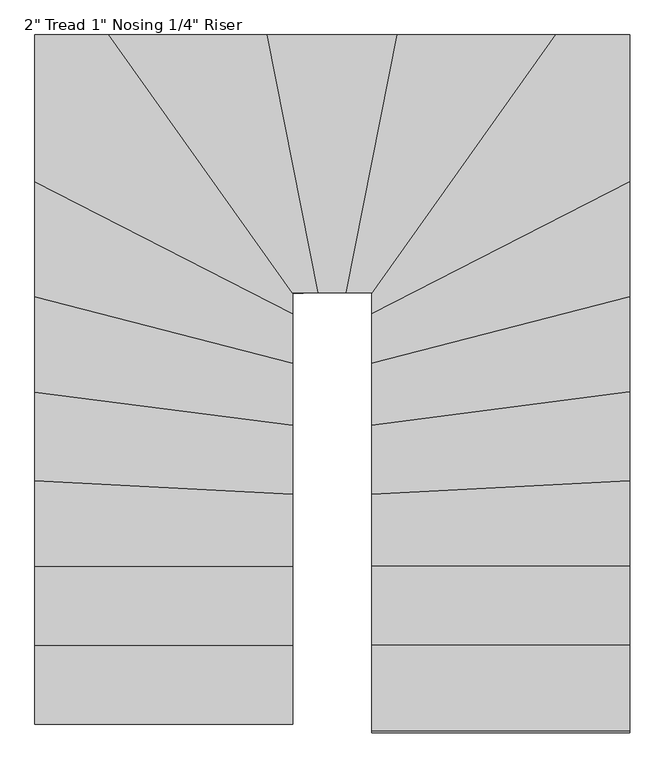
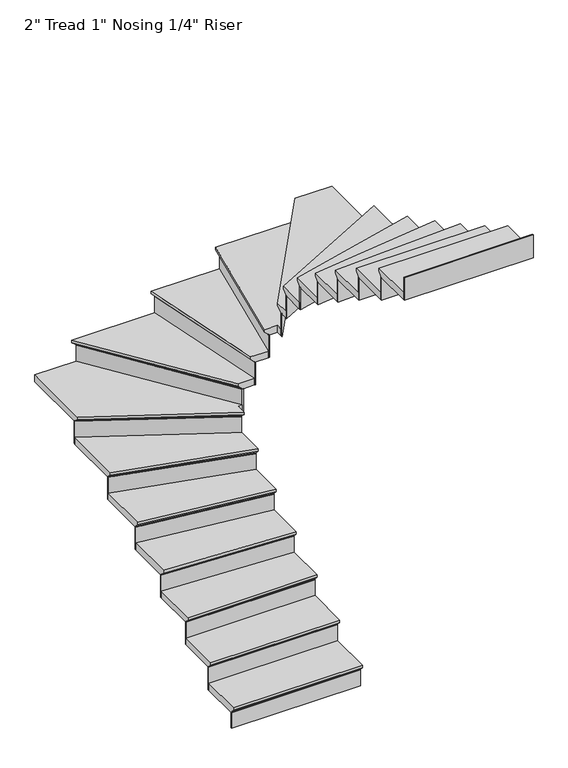
"""IFC4 building model written with IfcOpenShell, lengths in millimetres: stair flight geometry."""

from ifc_helpers import new_model, si_unit, origin, place, context, project, spatial, faceted_brep, source, transform, mapped, element, save


def stair_flight_3c83121e(model_context):
    return source(origin(), model_context, "Body", "Brep", [
        faceted_brep([(-12408.1357228, 11608.7303252, 150.2833333), (-12408.1357228, 11608.7303252, 169.3333333), (-13322.5357228, 11608.7303252, 169.3333333), (-13322.5357228, 11608.7303252, 150.2833333), (-12408.1357228, 11634.1303252, 124.8833333), (-13322.5357228, 11634.1303252, 124.8833333), (-12408.1357228, 11913.5303252, 169.3333333), (-13322.5357228, 11913.5303252, 169.3333333), (-13322.5357228, 11634.1303252, 118.5333333), (-13322.5357228, 11913.5303252, 118.5333333), (-12408.1357228, 11913.5303252, 118.5333333), (-12408.1357228, 11634.1303252, 118.5333333)], [[[0, 1, 2, 3]], [[4, 0, 3, 5]], [[2, 1, 6, 7]], [[8, 9, 10, 11]], [[2, 7, 9, 8, 5, 3]], [[8, 11, 4, 5]], [[6, 1, 0, 4, 11, 10]], [[7, 6, 10, 9]]]),
        faceted_brep([(-12408.1357228, 11634.1303252, 118.5333333), (-12408.1357228, 11634.1303252, 0.0), (-12408.1357228, 11640.4803252, 0.0), (-12408.1357228, 11640.4803252, 118.5333333), (-13322.5357228, 11634.1303252, 118.5333333), (-13322.5357228, 11640.4803252, 118.5333333), (-13322.5357228, 11640.4803252, 0.0), (-13322.5357228, 11634.1303252, 0.0)], [[[0, 1, 2, 3]], [[4, 5, 6, 7]], [[1, 0, 4, 7]], [[2, 1, 7, 6]], [[3, 2, 6, 5]], [[0, 3, 5, 4]]]),
        faceted_brep([(-12408.1357228, 11913.5303252, 287.8666667), (-12408.1357228, 11913.5303252, 118.5333333), (-12408.1357228, 11919.8803252, 118.5333333), (-12408.1357228, 11919.8803252, 287.8666667), (-13322.5357228, 11913.5303252, 287.8666667), (-13322.5357228, 11919.8803252, 287.8666667), (-13322.5357228, 11919.8803252, 118.5333333), (-13322.5357228, 11913.5303252, 118.5333333)], [[[0, 1, 2, 3]], [[4, 5, 6, 7]], [[1, 0, 4, 7]], [[2, 1, 7, 6]], [[3, 2, 6, 5]], [[0, 3, 5, 4]]]),
        faceted_brep([(-13322.5357228, 11888.1303252, 338.6666667), (-12408.1357228, 11888.1303252, 338.6666667), (-12408.1357228, 12192.9303252, 338.6666667), (-13322.5357228, 12192.9303252, 338.6666667), (-13322.5357228, 11913.5303252, 287.8666667), (-13322.5357228, 12192.9303252, 287.8666667), (-12408.1357228, 12192.9303252, 287.8666667), (-12408.1357228, 11913.5303252, 287.8666667), (-13322.5357228, 11913.5303252, 294.2166667), (-13322.5357228, 11888.1303252, 319.6166667), (-12408.1357228, 11913.5303252, 294.2166667), (-12408.1357228, 11888.1303252, 319.6166667)], [[[0, 1, 2, 3]], [[4, 5, 6, 7]], [[0, 3, 5, 4, 8, 9]], [[4, 7, 10, 8]], [[2, 1, 11, 10, 7, 6]], [[3, 2, 6, 5]], [[11, 1, 0, 9]], [[10, 11, 9, 8]]]),
        faceted_brep([(-12408.1357228, 12192.9303252, 457.2), (-12408.1357228, 12192.9303252, 287.8666667), (-12408.1357228, 12199.2803252, 287.8666667), (-12408.1357228, 12199.2803252, 457.2), (-13322.5357228, 12192.9303252, 457.2), (-13322.5357228, 12199.2803252, 457.2), (-13322.5357228, 12199.2803252, 287.8666667), (-13322.5357228, 12192.9303252, 287.8666667)], [[[0, 1, 2, 3]], [[4, 5, 6, 7]], [[1, 0, 4, 7]], [[2, 1, 7, 6]], [[3, 2, 6, 5]], [[0, 3, 5, 4]]]),
        faceted_brep([(-13322.5357228, 12167.5303252, 508.0), (-12408.1357228, 12167.5303252, 508.0), (-12408.1357228, 12448.5974867, 508.0), (-13322.5357228, 12496.1317571, 508.0), (-13322.5357228, 12192.9303252, 457.2), (-13322.5357228, 12496.1317571, 457.2), (-12408.1357228, 12448.5974867, 457.2), (-12408.1357228, 12192.9303252, 457.2), (-13322.5357228, 12192.9303252, 463.55), (-13322.5357228, 12167.5303252, 488.95), (-12408.1357228, 12192.9303252, 463.55), (-12408.1357228, 12167.5303252, 488.95)], [[[0, 1, 2, 3]], [[4, 5, 6, 7]], [[0, 3, 5, 4, 8, 9]], [[4, 7, 10, 8]], [[2, 1, 11, 10, 7, 6]], [[3, 2, 6, 5]], [[11, 1, 0, 9]], [[10, 11, 9, 8]]]),
        faceted_brep([(-12408.1357228, 12448.5974867, 626.5333333), (-12408.1357228, 12448.5974867, 457.2), (-12408.1357228, 12454.9560609, 457.2), (-12408.1357228, 12454.9560609, 626.5333333), (-13322.5357228, 12496.1317571, 626.5333333), (-13322.5357228, 12502.4903313, 626.5333333), (-13322.5357228, 12502.4903313, 457.2), (-13322.5357228, 12496.1317571, 457.2)], [[[0, 1, 2, 3]], [[4, 5, 6, 7]], [[1, 0, 4, 7]], [[2, 1, 7, 6]], [[3, 2, 6, 5]], [[0, 3, 5, 4]]]),
        faceted_brep([(-13322.5357228, 12470.6974605, 677.3333333), (-12408.1357228, 12423.16319, 677.3333333), (-12408.1357228, 12692.7641865, 677.3333333), (-13322.5357228, 12811.1202382, 677.3333333), (-13322.5357228, 12496.1317571, 626.5333333), (-13322.5357228, 12811.1202382, 626.5333333), (-12408.1357228, 12692.7641865, 626.5333333), (-12408.1357228, 12448.5974867, 626.5333333), (-13322.5357228, 12496.1317571, 632.8833333), (-13322.5357228, 12470.6974605, 658.2833333), (-12408.1357228, 12448.5974867, 632.8833333), (-12408.1357228, 12423.16319, 658.2833333)], [[[0, 1, 2, 3]], [[4, 5, 6, 7]], [[0, 3, 5, 4, 8, 9]], [[4, 7, 10, 8]], [[2, 1, 11, 10, 7, 6]], [[3, 2, 6, 5]], [[11, 1, 0, 9]], [[10, 11, 9, 8]]]),
        faceted_brep([(-12408.1357228, 12692.7641865, 795.8666667), (-12408.1357228, 12692.7641865, 626.5333333), (-12408.1357228, 12699.1671583, 626.5333333), (-12408.1357228, 12699.1671583, 795.8666667), (-13322.5357228, 12811.1202382, 795.8666667), (-13322.5357228, 12817.52321, 795.8666667), (-13322.5357228, 12817.52321, 626.5333333), (-13322.5357228, 12811.1202382, 626.5333333)], [[[0, 1, 2, 3]], [[4, 5, 6, 7]], [[1, 0, 4, 7]], [[2, 1, 7, 6]], [[3, 2, 6, 5]], [[0, 3, 5, 4]]]),
        faceted_brep([(-13322.5357228, 12785.5083511, 846.6666667), (-12408.1357228, 12667.1522994, 846.6666667), (-12408.1357228, 12914.391409, 846.6666667), (-13322.5357228, 13149.5218564, 846.6666667), (-13322.5357228, 12811.1202382, 795.8666667), (-13322.5357228, 13149.5218564, 795.8666667), (-12408.1357228, 12914.391409, 795.8666667), (-12408.1357228, 12692.7641865, 795.8666667), (-13322.5357228, 12811.1202382, 802.2166667), (-13322.5357228, 12785.5083511, 827.6166667), (-12408.1357228, 12692.7641865, 802.2166667), (-12408.1357228, 12667.1522994, 827.6166667)], [[[0, 1, 2, 3]], [[4, 5, 6, 7]], [[0, 3, 5, 4, 8, 9]], [[4, 7, 10, 8]], [[2, 1, 11, 10, 7, 6]], [[3, 2, 6, 5]], [[11, 1, 0, 9]], [[10, 11, 9, 8]]]),
        faceted_brep([(-12408.1357228, 12914.391409, 965.2), (-12408.1357228, 12914.391409, 795.8666667), (-12408.1357228, 12920.9479859, 795.8666667), (-12408.1357228, 12920.9479859, 965.2), (-13322.5357228, 13149.5218564, 965.2), (-13322.5357228, 13156.0784333, 965.2), (-13322.5357228, 13156.0784333, 795.8666667), (-13322.5357228, 13149.5218564, 795.8666667)], [[[0, 1, 2, 3]], [[4, 5, 6, 7]], [[1, 0, 4, 7]], [[2, 1, 7, 6]], [[3, 2, 6, 5]], [[0, 3, 5, 4]]]),
        faceted_brep([(-13322.5357228, 13123.295549, 1016.0), (-12408.1357228, 12888.1651015, 1016.0), (-12408.1357228, 13090.7380451, 1016.0), (-13322.5357228, 13559.5626664, 1016.0), (-13322.5357228, 13149.5218564, 965.2), (-13322.5357228, 13559.5626664, 965.2), (-12408.1357228, 13090.7380451, 965.2), (-12408.1357228, 12914.391409, 965.2), (-13322.5357228, 13149.5218564, 971.55), (-13322.5357228, 13123.295549, 996.95), (-12408.1357228, 12914.391409, 971.55), (-12408.1357228, 12888.1651015, 996.95)], [[[0, 1, 2, 3]], [[4, 5, 6, 7]], [[0, 3, 5, 4, 8, 9]], [[4, 7, 10, 8]], [[2, 1, 11, 10, 7, 6]], [[3, 2, 6, 5]], [[11, 1, 0, 9]], [[10, 11, 9, 8]]]),
        faceted_brep([(-12408.1357228, 13090.7380451, 1134.5333333), (-12408.1357228, 13090.7380451, 965.2), (-12408.1357228, 13097.8740282, 965.2), (-12408.1357228, 13097.8740282, 1134.5333333), (-13322.5357228, 13559.5626664, 1134.5333333), (-13322.5357228, 13566.6986496, 1134.5333333), (-13322.5357228, 13566.6986496, 965.2), (-13322.5357228, 13559.5626664, 965.2)], [[[0, 1, 2, 3]], [[4, 5, 6, 7]], [[1, 0, 4, 7]], [[2, 1, 7, 6]], [[3, 2, 6, 5]], [[0, 3, 5, 4]]]),
        faceted_brep([(-13028.8545891, 14050.8620171, 1185.3333333), (-13322.5357228, 14050.8620171, 1185.3333333), (-13322.5357228, 13531.0187339, 1185.3333333), (-12408.1357228, 13062.1941126, 1185.3333333), (-12408.1357228, 13136.4620171, 1185.3333333), (-12378.5806399, 13136.4620171, 1185.3333333), (-13322.5357228, 14050.8620171, 1134.5333333), (-13028.8545891, 14050.8620171, 1134.5333333), (-12378.5806399, 13136.4620171, 1134.5333333), (-12408.1357228, 13136.4620171, 1134.5333333), (-12408.1357228, 13090.7380451, 1134.5333333), (-13322.5357228, 13559.5626664, 1134.5333333), (-13322.5357228, 13559.5626664, 1140.8833333), (-13322.5357228, 13531.0187339, 1166.2833333), (-12408.1357228, 13090.7380451, 1140.8833333), (-12408.1357228, 13062.1941126, 1166.2833333)], [[[0, 1, 2, 3, 4, 5]], [[6, 7, 8, 9, 10, 11]], [[1, 0, 7, 6]], [[2, 1, 6, 11, 12, 13]], [[11, 10, 14, 12]], [[4, 3, 15, 14, 10, 9]], [[5, 4, 9, 8]], [[0, 5, 8, 7]], [[15, 3, 2, 13]], [[14, 15, 13, 12]]]),
        faceted_brep([(-12378.5806399, 13136.4620171, 1303.8666667), (-12378.5806399, 13136.4620171, 1134.5333333), (-12370.7886651, 13136.4620171, 1134.5333333), (-12370.7886651, 13136.4620171, 1303.8666667), (-13028.8545891, 14050.8620171, 1303.8666667), (-13021.0626143, 14050.8620171, 1303.8666667), (-13021.0626143, 14050.8620171, 1134.5333333), (-13028.8545891, 14050.8620171, 1134.5333333)], [[[0, 1, 2, 3]], [[4, 5, 6, 7]], [[1, 0, 4, 7]], [[2, 1, 7, 6]], [[3, 2, 6, 5]], [[0, 3, 5, 4]]]),
        faceted_brep([(-13060.0224883, 14050.8620171, 1354.6666667), (-12409.7485391, 13136.4620171, 1354.6666667), (-12292.1265529, 13136.4620171, 1354.6666667), (-12472.3674092, 14050.8620171, 1354.6666667), (-13028.8545891, 14050.8620171, 1303.8666667), (-12472.3674092, 14050.8620171, 1303.8666667), (-12292.1265529, 13136.4620171, 1303.8666667), (-12378.5806399, 13136.4620171, 1303.8666667), (-13028.8545891, 14050.8620171, 1310.2166667), (-13060.0224883, 14050.8620171, 1335.6166667), (-12378.5806399, 13136.4620171, 1310.2166667), (-12409.7485391, 13136.4620171, 1335.6166667)], [[[0, 1, 2, 3]], [[4, 5, 6, 7]], [[0, 3, 5, 4, 8, 9]], [[4, 7, 10, 8]], [[2, 1, 11, 10, 7, 6]], [[3, 2, 6, 5]], [[11, 1, 0, 9]], [[10, 11, 9, 8]]]),
        faceted_brep([(-12292.1265529, 13136.4620171, 1473.2), (-12292.1265529, 13136.4620171, 1303.8666667), (-12285.6543674, 13136.4620171, 1303.8666667), (-12285.6543674, 13136.4620171, 1473.2), (-12472.3674092, 14050.8620171, 1473.2), (-12465.8952238, 14050.8620171, 1473.2), (-12465.8952238, 14050.8620171, 1303.8666667), (-12472.3674092, 14050.8620171, 1303.8666667)], [[[0, 1, 2, 3]], [[4, 5, 6, 7]], [[1, 0, 4, 7]], [[2, 1, 7, 6]], [[3, 2, 6, 5]], [[0, 3, 5, 4]]]),
        faceted_brep([(-12498.2561509, 14050.8620171, 1524.0), (-12318.0152946, 13136.4620171, 1524.0), (-12192.9674092, 13136.4620171, 1524.0), (-12012.7265529, 14050.8620171, 1524.0), (-12472.3674092, 14050.8620171, 1473.2), (-12012.7265529, 14050.8620171, 1473.2), (-12192.9674092, 13136.4620171, 1473.2), (-12292.1265529, 13136.4620171, 1473.2), (-12472.3674092, 14050.8620171, 1479.55), (-12498.2561509, 14050.8620171, 1504.95), (-12292.1265529, 13136.4620171, 1479.55), (-12318.0152946, 13136.4620171, 1504.95)], [[[0, 1, 2, 3]], [[4, 5, 6, 7]], [[0, 3, 5, 4, 8, 9]], [[4, 7, 10, 8]], [[2, 1, 11, 10, 7, 6]], [[3, 2, 6, 5]], [[11, 1, 0, 9]], [[10, 11, 9, 8]]]),
        faceted_brep([(-12192.9674092, 13136.4620171, 1642.5333333), (-12192.9674092, 13136.4620171, 1473.2), (-12186.4952238, 13136.4620171, 1473.2), (-12186.4952238, 13136.4620171, 1642.5333333), (-12012.7265529, 14050.8620171, 1642.5333333), (-12006.2543674, 14050.8620171, 1642.5333333), (-12006.2543674, 14050.8620171, 1473.2), (-12012.7265529, 14050.8620171, 1473.2)], [[[0, 1, 2, 3]], [[4, 5, 6, 7]], [[1, 0, 4, 7]], [[2, 1, 7, 6]], [[3, 2, 6, 5]], [[0, 3, 5, 4]]]),
        faceted_brep([(-12038.6152946, 14050.8620171, 1693.3333333), (-12218.8561509, 13136.4620171, 1693.3333333), (-12128.7357228, 13136.4620171, 1693.3333333), (-12128.7357228, 13090.3665426, 1693.3333333), (-11445.6810581, 14050.8620171, 1693.3333333), (-12012.7265529, 14050.8620171, 1642.5333333), (-11445.6810581, 14050.8620171, 1642.5333333), (-12128.7357228, 13090.3665426, 1642.5333333), (-12128.7357228, 13136.4620171, 1642.5333333), (-12192.9674092, 13136.4620171, 1642.5333333), (-12012.7265529, 14050.8620171, 1648.8833333), (-12038.6152946, 14050.8620171, 1674.2833333), (-12192.9674092, 13136.4620171, 1648.8833333), (-12218.8561509, 13136.4620171, 1674.2833333)], [[[0, 1, 2, 3, 4]], [[5, 6, 7, 8, 9]], [[0, 4, 6, 5, 10, 11]], [[5, 9, 12, 10]], [[2, 1, 13, 12, 9, 8]], [[3, 2, 8, 7]], [[4, 3, 7, 6]], [[13, 1, 0, 11]], [[12, 13, 11, 10]]]),
        faceted_brep([(-12128.7357228, 13090.3665426, 1811.8666667), (-12128.7357228, 13090.3665426, 1642.5333333), (-12128.7357228, 13079.4096501, 1642.5333333), (-12128.7357228, 13079.4096501, 1811.8666667), (-11445.6810581, 14050.8620171, 1811.8666667), (-11437.8890833, 14050.8620171, 1811.8666667), (-11437.8890833, 14050.8620171, 1642.5333333), (-11445.6810581, 14050.8620171, 1642.5333333)], [[[0, 1, 2, 3]], [[4, 5, 6, 7]], [[1, 0, 4, 7]], [[2, 1, 7, 6]], [[3, 2, 6, 5]], [[0, 3, 5, 4]]]),
        faceted_brep([(-11214.3357228, 13502.4748013, 1862.6666667), (-11214.3357228, 14050.8620171, 1862.6666667), (-11476.8489573, 14050.8620171, 1862.6666667), (-12128.7357228, 13134.1941126, 1862.6666667), (-12128.7357228, 13033.65018, 1862.6666667), (-11214.3357228, 14050.8620171, 1811.8666667), (-11214.3357228, 13502.4748013, 1811.8666667), (-12128.7357228, 13033.65018, 1811.8666667), (-12128.7357228, 13090.3665426, 1811.8666667), (-11445.6810581, 14050.8620171, 1811.8666667), (-11445.6810581, 14050.8620171, 1818.2166667), (-11476.8489573, 14050.8620171, 1843.6166667), (-12128.7357228, 13090.3665426, 1818.2166667), (-12128.7357228, 13134.1941126, 1843.6166667)], [[[0, 1, 2, 3, 4]], [[5, 6, 7, 8, 9]], [[1, 0, 6, 5]], [[2, 1, 5, 9, 10, 11]], [[9, 8, 12, 10]], [[4, 3, 13, 12, 8, 7]], [[0, 4, 7, 6]], [[13, 3, 2, 11]], [[12, 13, 11, 10]]]),
        faceted_brep([(-12128.7357228, 13033.65018, 1981.2), (-12128.7357228, 13033.65018, 1811.8666667), (-12128.7357228, 13026.5141969, 1811.8666667), (-12128.7357228, 13026.5141969, 1981.2), (-11214.3357228, 13502.4748013, 1981.2), (-11214.3357228, 13495.3388182, 1981.2), (-11214.3357228, 13495.3388182, 1811.8666667), (-11214.3357228, 13502.4748013, 1811.8666667)], [[[0, 1, 2, 3]], [[4, 5, 6, 7]], [[1, 0, 4, 7]], [[2, 1, 7, 6]], [[3, 2, 6, 5]], [[0, 3, 5, 4]]]),
        faceted_brep([(-11214.3357228, 13531.0187339, 2032.0), (-12128.7357228, 13062.1941126, 2032.0), (-12128.7357228, 12861.9387941, 2032.0), (-11214.3357228, 13097.0692415, 2032.0), (-11214.3357228, 13502.4748013, 1981.2), (-11214.3357228, 13097.0692415, 1981.2), (-12128.7357228, 12861.9387941, 1981.2), (-12128.7357228, 13033.65018, 1981.2), (-11214.3357228, 13502.4748013, 1987.55), (-11214.3357228, 13531.0187339, 2012.95), (-12128.7357228, 13033.65018, 1987.55), (-12128.7357228, 13062.1941126, 2012.95)], [[[0, 1, 2, 3]], [[4, 5, 6, 7]], [[0, 3, 5, 4, 8, 9]], [[4, 7, 10, 8]], [[2, 1, 11, 10, 7, 6]], [[3, 2, 6, 5]], [[11, 1, 0, 9]], [[10, 11, 9, 8]]]),
        faceted_brep([(-12128.7357228, 12861.9387941, 2150.5333333), (-12128.7357228, 12861.9387941, 1981.2), (-12128.7357228, 12855.3822172, 1981.2), (-12128.7357228, 12855.3822172, 2150.5333333), (-11214.3357228, 13097.0692415, 2150.5333333), (-11214.3357228, 13090.5126646, 2150.5333333), (-11214.3357228, 13090.5126646, 1981.2), (-11214.3357228, 13097.0692415, 1981.2)], [[[0, 1, 2, 3]], [[4, 5, 6, 7]], [[1, 0, 4, 7]], [[2, 1, 7, 6]], [[3, 2, 6, 5]], [[0, 3, 5, 4]]]),
        faceted_brep([(-11214.3357228, 13123.295549, 2201.3333333), (-12128.7357228, 12888.1651015, 2201.3333333), (-12128.7357228, 12641.5404123, 2201.3333333), (-11214.3357228, 12759.896464, 2201.3333333), (-11214.3357228, 13097.0692415, 2150.5333333), (-11214.3357228, 12759.896464, 2150.5333333), (-12128.7357228, 12641.5404123, 2150.5333333), (-12128.7357228, 12861.9387941, 2150.5333333), (-11214.3357228, 13097.0692415, 2156.8833333), (-11214.3357228, 13123.295549, 2182.2833333), (-12128.7357228, 12861.9387941, 2156.8833333), (-12128.7357228, 12888.1651015, 2182.2833333)], [[[0, 1, 2, 3]], [[4, 5, 6, 7]], [[0, 3, 5, 4, 8, 9]], [[4, 7, 10, 8]], [[2, 1, 11, 10, 7, 6]], [[3, 2, 6, 5]], [[11, 1, 0, 9]], [[10, 11, 9, 8]]]),
        faceted_brep([(-12128.7357228, 12641.5404123, 2319.8666667), (-12128.7357228, 12641.5404123, 2150.5333333), (-12128.7357228, 12635.1374405, 2150.5333333), (-12128.7357228, 12635.1374405, 2319.8666667), (-11214.3357228, 12759.896464, 2319.8666667), (-11214.3357228, 12753.4934922, 2319.8666667), (-11214.3357228, 12753.4934922, 2150.5333333), (-11214.3357228, 12759.896464, 2150.5333333)], [[[0, 1, 2, 3]], [[4, 5, 6, 7]], [[1, 0, 4, 7]], [[2, 1, 7, 6]], [[3, 2, 6, 5]], [[0, 3, 5, 4]]]),
        faceted_brep([(-11214.3357228, 12785.5083511, 2370.6666667), (-12128.7357228, 12667.1522994, 2370.6666667), (-12128.7357228, 12397.7288934, 2370.6666667), (-11214.3357228, 12445.2631638, 2370.6666667), (-11214.3357228, 12759.896464, 2319.8666667), (-11214.3357228, 12445.2631638, 2319.8666667), (-12128.7357228, 12397.7288934, 2319.8666667), (-12128.7357228, 12641.5404123, 2319.8666667), (-11214.3357228, 12759.896464, 2326.2166667), (-11214.3357228, 12785.5083511, 2351.6166667), (-12128.7357228, 12641.5404123, 2326.2166667), (-12128.7357228, 12667.1522994, 2351.6166667)], [[[0, 1, 2, 3]], [[4, 5, 6, 7]], [[0, 3, 5, 4, 8, 9]], [[4, 7, 10, 8]], [[2, 1, 11, 10, 7, 6]], [[3, 2, 6, 5]], [[11, 1, 0, 9]], [[10, 11, 9, 8]]]),
        faceted_brep([(-12128.7357228, 12397.7288934, 2489.2), (-12128.7357228, 12397.7288934, 2319.8666667), (-12128.7357228, 12391.3703192, 2319.8666667), (-12128.7357228, 12391.3703192, 2489.2), (-11214.3357228, 12445.2631638, 2489.2), (-11214.3357228, 12438.9045896, 2489.2), (-11214.3357228, 12438.9045896, 2319.8666667), (-11214.3357228, 12445.2631638, 2319.8666667)], [[[0, 1, 2, 3]], [[4, 5, 6, 7]], [[1, 0, 4, 7]], [[2, 1, 7, 6]], [[3, 2, 6, 5]], [[0, 3, 5, 4]]]),
        faceted_brep([(-11214.3357228, 12470.6974605, 2540.0), (-12128.7357228, 12423.16319, 2540.0), (-12128.7357228, 12142.1303252, 2540.0), (-11214.3357228, 12142.1303252, 2540.0), (-11214.3357228, 12445.2631638, 2489.2), (-11214.3357228, 12142.1303252, 2489.2), (-12128.7357228, 12142.1303252, 2489.2), (-12128.7357228, 12397.7288934, 2489.2), (-11214.3357228, 12445.2631638, 2495.55), (-11214.3357228, 12470.6974605, 2520.95), (-12128.7357228, 12397.7288934, 2495.55), (-12128.7357228, 12423.16319, 2520.95)], [[[0, 1, 2, 3]], [[4, 5, 6, 7]], [[0, 3, 5, 4, 8, 9]], [[4, 7, 10, 8]], [[2, 1, 11, 10, 7, 6]], [[3, 2, 6, 5]], [[11, 1, 0, 9]], [[10, 11, 9, 8]]]),
        faceted_brep([(-12128.7357228, 12142.1303252, 2658.5333333), (-12128.7357228, 12142.1303252, 2489.2), (-12128.7357228, 12135.7803252, 2489.2), (-12128.7357228, 12135.7803252, 2658.5333333), (-11214.3357228, 12142.1303252, 2658.5333333), (-11214.3357228, 12135.7803252, 2658.5333333), (-11214.3357228, 12135.7803252, 2489.2), (-11214.3357228, 12142.1303252, 2489.2)], [[[0, 1, 2, 3]], [[4, 5, 6, 7]], [[1, 0, 4, 7]], [[2, 1, 7, 6]], [[3, 2, 6, 5]], [[0, 3, 5, 4]]]),
        faceted_brep([(-11214.3357228, 12167.5303252, 2709.3333333), (-12128.7357228, 12167.5303252, 2709.3333333), (-12128.7357228, 11862.7303252, 2709.3333333), (-11214.3357228, 11862.7303252, 2709.3333333), (-11214.3357228, 12142.1303252, 2658.5333333), (-11214.3357228, 11862.7303252, 2658.5333333), (-12128.7357228, 11862.7303252, 2658.5333333), (-12128.7357228, 12142.1303252, 2658.5333333), (-11214.3357228, 12142.1303252, 2664.8833333), (-11214.3357228, 12167.5303252, 2690.2833333), (-12128.7357228, 12142.1303252, 2664.8833333), (-12128.7357228, 12167.5303252, 2690.2833333)], [[[0, 1, 2, 3]], [[4, 5, 6, 7]], [[0, 3, 5, 4, 8, 9]], [[4, 7, 10, 8]], [[2, 1, 11, 10, 7, 6]], [[3, 2, 6, 5]], [[11, 1, 0, 9]], [[10, 11, 9, 8]]]),
        faceted_brep([(-12128.7357228, 11862.7303252, 2827.8666667), (-12128.7357228, 11862.7303252, 2658.5333333), (-12128.7357228, 11856.3803252, 2658.5333333), (-12128.7357228, 11856.3803252, 2827.8666667), (-11214.3357228, 11862.7303252, 2827.8666667), (-11214.3357228, 11856.3803252, 2827.8666667), (-11214.3357228, 11856.3803252, 2658.5333333), (-11214.3357228, 11862.7303252, 2658.5333333)], [[[0, 1, 2, 3]], [[4, 5, 6, 7]], [[1, 0, 4, 7]], [[2, 1, 7, 6]], [[3, 2, 6, 5]], [[0, 3, 5, 4]]]),
        faceted_brep([(-12128.7357228, 11583.3303252, 2997.2), (-12128.7357228, 11583.3303252, 2827.8666667), (-12128.7357228, 11576.9803252, 2827.8666667), (-12128.7357228, 11576.9803252, 2997.2), (-11214.3357228, 11583.3303252, 2997.2), (-11214.3357228, 11576.9803252, 2997.2), (-11214.3357228, 11576.9803252, 2827.8666667), (-11214.3357228, 11583.3303252, 2827.8666667)], [[[0, 1, 2, 3]], [[4, 5, 6, 7]], [[1, 0, 4, 7]], [[2, 1, 7, 6]], [[3, 2, 6, 5]], [[0, 3, 5, 4]]]),
        faceted_brep([(-11214.3357228, 11888.1303252, 2878.6666667), (-12128.7357228, 11888.1303252, 2878.6666667), (-12128.7357228, 11583.3303252, 2878.6666667), (-11214.3357228, 11583.3303252, 2878.6666667), (-11214.3357228, 11862.7303252, 2827.8666667), (-11214.3357228, 11583.3303252, 2827.8666667), (-12128.7357228, 11583.3303252, 2827.8666667), (-12128.7357228, 11862.7303252, 2827.8666667), (-11214.3357228, 11862.7303252, 2834.2166667), (-11214.3357228, 11888.1303252, 2859.6166667), (-12128.7357228, 11862.7303252, 2834.2166667), (-12128.7357228, 11888.1303252, 2859.6166667)], [[[0, 1, 2, 3]], [[4, 5, 6, 7]], [[0, 3, 5, 4, 8, 9]], [[4, 7, 10, 8]], [[2, 1, 11, 10, 7, 6]], [[3, 2, 6, 5]], [[11, 1, 0, 9]], [[10, 11, 9, 8]]]),
    ])


if __name__ == "__main__":
    model = new_model("IFC4")
    model_context = context("Model", 3, world=origin())
    ifc_project = project(units=[si_unit("LENGTHUNIT", "METRE", prefix="MILLI")], contexts=[model_context])
    site = spatial("IfcSite", under=ifc_project)
    building = spatial("IfcBuilding", under=site)
    placement = place(None, origin())
    stair_flight_shape = stair_flight_3c83121e(model_context)
    element("IfcStairFlight", 1, ObjectType="2\" Tread 1\" Nosing 1/4\" Riser", at=placement, inside=building, context=model_context, shape_type="MappedRepresentation", body=[
        mapped(stair_flight_shape, transform((0.0, 0.0, 0.0), x_axis=(1.0, 0.0, 0.0), y_axis=(0.0, 1.0, 0.0), z_axis=(0.0, 0.0, 1.0))),
    ])
    save(model, "model.ifc")
